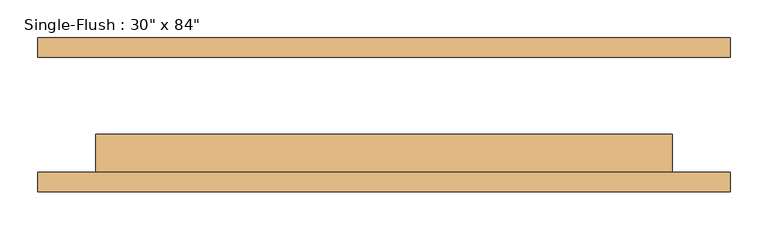
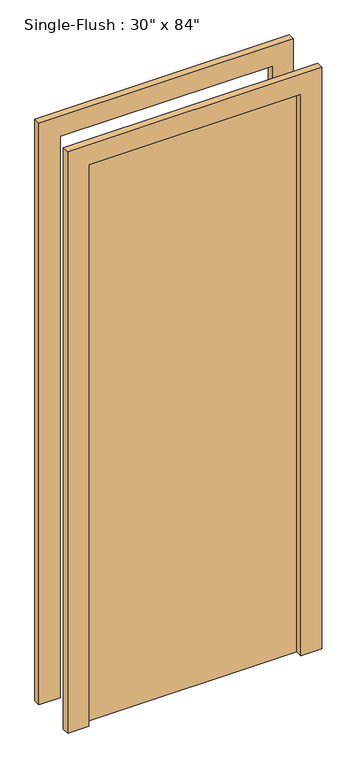
"""IFC4 building model written with IfcOpenShell, lengths in millimetres: door geometry."""

from ifc_helpers import new_model, si_unit, frame, origin, origin_with_axes, place, context, project, spatial, polyline, outline, extrude, source, transform, mapped, element, save


def door_e2b13fe9(model_context):
    return source(origin(), model_context, "Body", "SweptSolid", [
        extrude(outline(polyline([(2209.8, -457.2), (0.0, -457.2), (0.0, -381.0), (2133.6, -381.0), (2133.6, 381.0), (0.0, 381.0), (0.0, 457.2), (2209.8, 457.2), (2209.8, -457.2)])), frame((0.0, -101.6, 0.0), z_axis=(0.0, 1.0, 0.0), x_axis=(0.0, 0.0, 1.0)), (0.0, 0.0, 1.0), 25.4),
        extrude(outline(polyline([(2209.8, 457.2), (2209.8, -457.2), (0.0, -457.2), (0.0, -381.0), (2133.6, -381.0), (2133.6, 381.0), (0.0, 381.0), (0.0, 457.2), (2209.8, 457.2)])), frame((0.0, 76.2, 0.0), z_axis=(0.0, 1.0, 0.0), x_axis=(0.0, 0.0, 1.0)), (0.0, 0.0, 1.0), 25.4),
        extrude(outline(polyline([(381.0, -25.4), (381.0, -76.2), (-381.0, -76.2), (-381.0, -25.4), (381.0, -25.4)])), origin_with_axes(), (0.0, 0.0, 1.0), 2133.6),
    ])


if __name__ == "__main__":
    model = new_model("IFC4")
    model_context = context("Model", 3, world=origin())
    ifc_project = project(units=[si_unit("LENGTHUNIT", "METRE", prefix="MILLI")], contexts=[model_context])
    site = spatial("IfcSite", under=ifc_project)
    building = spatial("IfcBuilding", under=site)
    placement = place(None, origin())
    door_shape = door_e2b13fe9(model_context)
    element("IfcDoor", 1, ObjectType="Single-Flush : 30\" x 84\"", at=placement, inside=building, context=model_context, shape_type="MappedRepresentation", body=[
        mapped(door_shape, transform((0.0, 0.0, 0.0), x_axis=(1.0, 0.0, 0.0), y_axis=(0.0, 1.0, 0.0), z_axis=(0.0, 0.0, 1.0))),
    ])
    save(model, "model.ifc")

# Revit data of these elements
# Type "Single-Flush : 30\" x 84\""
#   Type Mark = "4"
#   Construction Type Id = "MDOOR"
#   Assembly Code = "C1020"
#   Analytic Construction = "Metal"
#   Thickness = 0' - 2"
#   Heat Transfer Coefficient (U) = 0.651978 BTU/(h·ft²·°F)
#   Height = 7' - 0"
#   Trim Projection Ext = 0' - 1"
#   Trim Projection Int = 0' - 1"
#   Trim Width = 0' - 3"
#   Width = 2' - 6"
#   Define Thermal Properties by = 1
#   Define Thermal Properties by = 1
#   Door Material = Door - Panel
#   Frame Material = Door - Frame
#   Visual Light Transmittance = 0
#   Solar Heat Gain Coefficient = 0
#   Function = (empty or 0)
#   Wall Closure = (empty or 0)
# Element 1 (IfcDoor, "Single-Flush : 30\" x 84\"")
#   Materials on its faces: "Door - Frame", "Door - Panel"
# Materials
#   "Door - Panel": class "Wood", colour RGB 210 159 95, transparency 0, Cost = 0
#   "Door - Frame": colour RGB 118 70 51, transparency 0, Cost = 0
